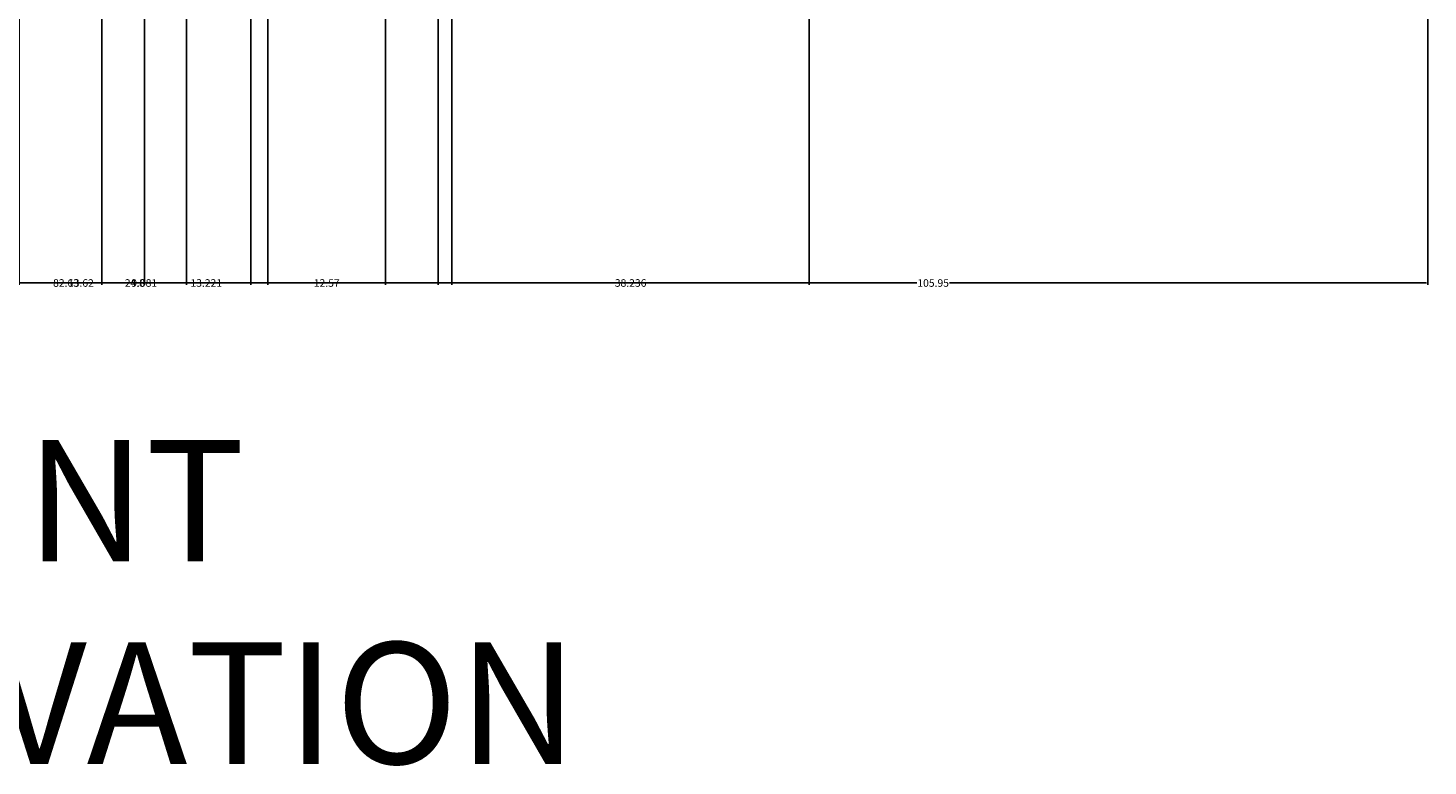
# Model space of a CAD drawing. Units: inches. Extents: x 69 to 650, y -16 to 573.
# Tile 6 of 26: x 345 to 495, y -16 to 63. Entities that reach past the tile are written whole.
import ezdxf

# ---------------------------------------------------------------- set-up
doc = ezdxf.new("R2010")
doc.units = ezdxf.units.IN
doc.header["$MEASUREMENT"] = 0
doc.layers.add('A-ANNO-DIMS', color=2, linetype='Continuous', lineweight=18)
doc.layers.add('A-ANNO-TEXT', color=7, linetype='Continuous', lineweight=25)
doc.styles.get("Standard").update_dxf_attribs({"font": 'arial.ttf'})
doc.dimstyles.get("Standard").update_dxf_attribs({"dimtxt": 0.8125, "dimasz": 0.18, "dimexe": 0.18, "dimexo": 0.0625, "dimgap": 0.09, "dimtad": 0, "dimtih": 1, "dimtoh": 1, "dimdec": 4, "dimzin": 0, "dimdsep": 46, "dimlunit": 4, "dimtxsty": 'Standard', "dimcen": 0.09, "dimadec": 0, "dimazin": 0, "dimtfac": 1, "dimtdec": 4, "dimtofl": 0, "dimtmove": 0, "dimatfit": 3, "dimfxl": 1, "dimtolj": 1, "dimtzin": 0, "dimarcsym": 0})

# ---------------------------------------------------------------- blocks, each defined once
blk = doc.blocks.new('*D30')
at = {"layer": 'A-ANNO-DIMS', "color": 0, "lineweight": -2, "transparency": 16777216}
for p, q in [((352.94, 174.2), (352.94, 35.35)), ((313.14, 87.92), (313.14, 35.35)), ((313.32, 35.53), (331.9, 35.53)), ((352.76, 35.53), (334.19, 35.53))]:
    blk.add_line(p, q, dxfattribs=at)
at = {"layer": 'A-ANNO-DIMS', "color": 0, "transparency": 16777216}
for points in [[(313.32, 35.56), (313.32, 35.5), (313.14, 35.53)], [(352.76, 35.56), (352.76, 35.5), (352.94, 35.53)]]:
    blk.add_solid(points, dxfattribs=at)
at = {"layer": 'Defpoints', "color": 0, "transparency": 16777216}
for p in [(352.94, 174.27), (313.14, 87.99), (352.94, 35.53)]:
    blk.add_point(p, dxfattribs=at)
at = {"layer": 'A-ANNO-DIMS', "color": 0, "transparency": 16777216, "insert": (333.04, 35.53), "char_height": 0.812, "attachment_point": 5}
blk.add_mtext('\\A1;39.8', dxfattribs=at)
blk = doc.blocks.new('*D31')
at = {"layer": 'A-ANNO-DIMS', "color": 0, "lineweight": -2, "transparency": 16777216}
for p, q in [((352.94, 174.2), (352.94, 35.35)), ((362.02, 87.87), (362.02, 35.35)), ((353.12, 35.53), (356.1, 35.53)), ((361.84, 35.53), (358.86, 35.53))]:
    blk.add_line(p, q, dxfattribs=at)
at = {"layer": 'A-ANNO-DIMS', "color": 0, "transparency": 16777216}
for points in [[(353.12, 35.56), (353.12, 35.5), (352.94, 35.53)], [(361.84, 35.56), (361.84, 35.5), (362.02, 35.53)]]:
    blk.add_solid(points, dxfattribs=at)
at = {"layer": 'Defpoints', "color": 0, "transparency": 16777216}
for p in [(352.94, 174.27), (362.02, 87.93), (362.02, 35.53)]:
    blk.add_point(p, dxfattribs=at)
at = {"layer": 'A-ANNO-DIMS', "color": 0, "transparency": 16777216, "insert": (357.48, 35.53), "char_height": 0.812, "attachment_point": 5}
blk.add_mtext('\\A1;9.081', dxfattribs=at)
blk = doc.blocks.new('*D32')
at = {"layer": 'A-ANNO-DIMS', "color": 0, "lineweight": -2, "transparency": 16777216}
for p, q in [((388.96, 87.87), (388.96, 35.35)), ((494.91, 87.87), (494.91, 35.35)), ((389.14, 35.53), (440.2, 35.53)), ((494.73, 35.53), (443.68, 35.53))]:
    blk.add_line(p, q, dxfattribs=at)
at = {"layer": 'A-ANNO-DIMS', "color": 0, "transparency": 16777216}
for points in [[(389.14, 35.56), (389.14, 35.5), (388.96, 35.53)], [(494.73, 35.56), (494.73, 35.5), (494.91, 35.53)]]:
    blk.add_solid(points, dxfattribs=at)
at = {"layer": 'Defpoints', "color": 0, "transparency": 16777216}
for p in [(388.96, 87.93), (494.91, 87.93), (494.91, 35.53)]:
    blk.add_point(p, dxfattribs=at)
at = {"layer": 'A-ANNO-DIMS', "color": 0, "transparency": 16777216, "insert": (441.94, 35.53), "char_height": 0.812, "attachment_point": 5}
blk.add_mtext('\\A1;105.95', dxfattribs=at)
blk = doc.blocks.new('*D38')
at = {"layer": 'A-ANNO-DIMS', "color": 0, "lineweight": -2, "transparency": 16777216}
for p, q in [((307.8, 384.84), (307.8, 35.35)), ((390.43, 384.84), (390.43, 35.35)), ((307.98, 35.53), (347.65, 35.53)), ((390.25, 35.53), (350.57, 35.53))]:
    blk.add_line(p, q, dxfattribs=at)
at = {"layer": 'A-ANNO-DIMS', "color": 0, "transparency": 16777216}
for points in [[(307.98, 35.56), (307.98, 35.5), (307.8, 35.53)], [(390.25, 35.56), (390.25, 35.5), (390.43, 35.53)]]:
    blk.add_solid(points, dxfattribs=at)
at = {"layer": 'Defpoints', "color": 0, "transparency": 16777216}
for p in [(307.8, 384.9), (390.43, 384.9), (390.43, 35.53)]:
    blk.add_point(p, dxfattribs=at)
at = {"layer": 'A-ANNO-DIMS', "color": 0, "transparency": 16777216, "insert": (349.11, 35.53), "char_height": 0.812, "attachment_point": 5}
blk.add_mtext('\\A1;82.63', dxfattribs=at)
blk = doc.blocks.new('*D39')
at = {"layer": 'A-ANNO-DIMS', "color": 0, "lineweight": -2, "transparency": 16777216}
for p, q in [((390.43, 384.84), (390.43, 35.35)), ((428.66, 372.93), (428.66, 35.35)), ((390.61, 35.53), (407.77, 35.53)), ((428.48, 35.53), (411.32, 35.53))]:
    blk.add_line(p, q, dxfattribs=at)
at = {"layer": 'A-ANNO-DIMS', "color": 0, "transparency": 16777216}
for points in [[(390.61, 35.56), (390.61, 35.5), (390.43, 35.53)], [(428.48, 35.56), (428.48, 35.5), (428.66, 35.53)]]:
    blk.add_solid(points, dxfattribs=at)
at = {"layer": 'Defpoints', "color": 0, "transparency": 16777216}
for p in [(390.43, 384.9), (428.66, 372.99), (428.66, 35.53)]:
    blk.add_point(p, dxfattribs=at)
at = {"layer": 'A-ANNO-DIMS', "color": 0, "transparency": 16777216, "insert": (409.55, 35.53), "char_height": 0.812, "attachment_point": 5}
blk.add_mtext('\\A1;38.236', dxfattribs=at)
blk = doc.blocks.new('*D65')
at = {"layer": 'A-ANNO-DIMS', "color": 0, "lineweight": -2, "transparency": 16777216}
for p, q in [((344.08, 393.8), (344.08, 35.35)), ((368.88, 393.8), (368.88, 35.35)), ((344.26, 35.53), (355.33, 35.53)), ((368.7, 35.53), (357.63, 35.53))]:
    blk.add_line(p, q, dxfattribs=at)
at = {"layer": 'A-ANNO-DIMS', "color": 0, "transparency": 16777216}
for points in [[(344.26, 35.56), (344.26, 35.5), (344.08, 35.53)], [(368.7, 35.56), (368.7, 35.5), (368.88, 35.53)]]:
    blk.add_solid(points, dxfattribs=at)
at = {"layer": 'Defpoints', "color": 0, "transparency": 16777216}
for p in [(344.08, 393.86), (368.88, 393.86), (368.88, 35.53)]:
    blk.add_point(p, dxfattribs=at)
at = {"layer": 'A-ANNO-DIMS', "color": 0, "transparency": 16777216, "insert": (356.48, 35.53), "char_height": 0.812, "attachment_point": 5}
blk.add_mtext('\\A1;24.8', dxfattribs=at)
blk = doc.blocks.new('*D69')
at = {"layer": 'A-ANNO-DIMS', "color": 0, "lineweight": -2, "transparency": 16777216}
for p, q in [((343.89, 263.46), (343.89, 35.35)), ((357.51, 263.46), (357.51, 35.35)), ((344.07, 35.53), (349.28, 35.53)), ((357.33, 35.53), (352.12, 35.53))]:
    blk.add_line(p, q, dxfattribs=at)
at = {"layer": 'A-ANNO-DIMS', "color": 0, "transparency": 16777216}
for points in [[(344.07, 35.56), (344.07, 35.5), (343.89, 35.53)], [(357.33, 35.56), (357.33, 35.5), (357.51, 35.53)]]:
    blk.add_solid(points, dxfattribs=at)
at = {"layer": 'Defpoints', "color": 0, "transparency": 16777216}
for p in [(343.89, 263.53), (357.51, 263.53), (357.51, 35.53)]:
    blk.add_point(p, dxfattribs=at)
at = {"layer": 'A-ANNO-DIMS', "color": 0, "transparency": 16777216, "insert": (350.7, 35.53), "char_height": 0.812, "attachment_point": 5}
blk.add_mtext('\\A1;13.62', dxfattribs=at)
blk = doc.blocks.new('*D70')
at = {"layer": 'A-ANNO-DIMS', "color": 0, "lineweight": -2, "transparency": 16777216}
for p, q in [((357.51, 263.46), (357.51, 35.35)), ((370.73, 263.46), (370.73, 35.35)), ((357.69, 35.53), (362.46, 35.53)), ((370.55, 35.53), (365.78, 35.53))]:
    blk.add_line(p, q, dxfattribs=at)
at = {"layer": 'A-ANNO-DIMS', "color": 0, "transparency": 16777216}
for points in [[(357.69, 35.56), (357.69, 35.5), (357.51, 35.53)], [(370.55, 35.56), (370.55, 35.5), (370.73, 35.53)]]:
    blk.add_solid(points, dxfattribs=at)
at = {"layer": 'Defpoints', "color": 0, "transparency": 16777216}
for p in [(357.51, 263.53), (370.73, 263.53), (370.73, 35.53)]:
    blk.add_point(p, dxfattribs=at)
at = {"layer": 'A-ANNO-DIMS', "color": 0, "transparency": 16777216, "insert": (364.12, 35.53), "char_height": 0.812, "attachment_point": 5}
blk.add_mtext('\\A1;13.221', dxfattribs=at)
blk = doc.blocks.new('*D71')
at = {"layer": 'A-ANNO-DIMS', "color": 0, "lineweight": -2, "transparency": 16777216}
for p, q in [((370.73, 263.46), (370.73, 35.35)), ((383.3, 263.46), (383.3, 35.35)), ((370.91, 35.53), (375.59, 35.53)), ((383.12, 35.53), (378.44, 35.53))]:
    blk.add_line(p, q, dxfattribs=at)
at = {"layer": 'A-ANNO-DIMS', "color": 0, "transparency": 16777216}
for points in [[(370.91, 35.56), (370.91, 35.5), (370.73, 35.53)], [(383.12, 35.56), (383.12, 35.5), (383.3, 35.53)]]:
    blk.add_solid(points, dxfattribs=at)
at = {"layer": 'Defpoints', "color": 0, "transparency": 16777216}
for p in [(370.73, 263.53), (383.3, 263.53), (383.3, 35.53)]:
    blk.add_point(p, dxfattribs=at)
at = {"layer": 'A-ANNO-DIMS', "color": 0, "transparency": 16777216, "insert": (377.02, 35.53), "char_height": 0.812, "attachment_point": 5}
blk.add_mtext('\\A1;12.57', dxfattribs=at)

msp = doc.modelspace()

# ---------------------------------------------------------------- texts
at = {"layer": 'A-ANNO-TEXT', "insert": (310.6022, 18.729), "char_height": 13, "attachment_point": 1}
msp.add_mtext_dynamic_manual_height_columns('FRONT ELEVATION', width=154.108417, gutter_width=1, heights=[0], dxfattribs=at)

# ---------------------------------------------------------------- dimensions: what is measured, and where the dimension line sits
at = {"layer": 'A-ANNO-DIMS'}
for base, p1, p2, override, picture, middle in [((368.881, 35.53), (344.0804, 393.8576), (368.881, 393.8576), {"dimdec": 1, "dimlfac": 1, "dimrnd": 0, "dimzin": 0, "dimdsep": 46, "dimlunit": 2}, '*D65', (356.4807, 35.53)), ((390.4291, 35.53), (307.7955, 384.8986), (390.4291, 384.8986), {"dimdec": 2, "dimlfac": 1, "dimrnd": 0, "dimzin": 0, "dimdsep": 46, "dimlunit": 2}, '*D38', (349.1123, 35.53)), ((428.6648, 35.53), (390.4291, 384.8986), (428.6648, 372.9907), {"dimdec": 3, "dimlfac": 1, "dimrnd": 0, "dimzin": 0, "dimdsep": 46, "dimlunit": 2}, '*D39', (409.547, 35.53)), ((357.5106, 35.53), (343.8902, 263.5253), (357.5106, 263.5253), {"dimdec": 2, "dimlfac": 1, "dimrnd": 0, "dimzin": 0, "dimdsep": 46, "dimlunit": 2}, '*D69', (350.7004, 35.53)), ((370.7319, 35.53), (357.5106, 263.5253), (370.7319, 263.5253), {"dimdec": 3, "dimlfac": 1, "dimrnd": 0, "dimzin": 0, "dimdsep": 46, "dimlunit": 2}, '*D70', (364.1213, 35.53)), ((383.3022, 35.53), (370.7319, 263.5253), (383.3022, 263.5253), {"dimdec": 2, "dimlfac": 1, "dimrnd": 0, "dimzin": 0, "dimdsep": 46, "dimlunit": 2}, '*D71', (377.0171, 35.53)), ((352.9415, 35.53), (313.1416, 87.985), (352.9415, 174.2666), {"dimdec": 1, "dimlfac": 1, "dimrnd": 0, "dimzin": 0, "dimdsep": 46, "dimlunit": 2}, '*D30', (333.0415, 35.53)), ((362.0229, 35.53), (352.9415, 174.2666), (362.0229, 87.93), {"dimdec": 3, "dimlfac": 1, "dimrnd": 0, "dimzin": 0, "dimdsep": 46, "dimlunit": 2}, '*D31', (357.4822, 35.53)), ((494.915, 35.53), (388.9646, 87.93), (494.915, 87.93), {"dimdec": 2, "dimlfac": 1, "dimrnd": 0, "dimzin": 0, "dimdsep": 46, "dimlunit": 2}, '*D32', (441.9398, 35.53))]:
    dim = msp.add_linear_dim(base=base, p1=p1, p2=p2, dimstyle='Standard', override=override, dxfattribs=at)
    dim.commit()
    dim.dimension.update_dxf_attribs({"geometry": picture, "text_midpoint": middle})

doc.saveas('drawing.dxf')
